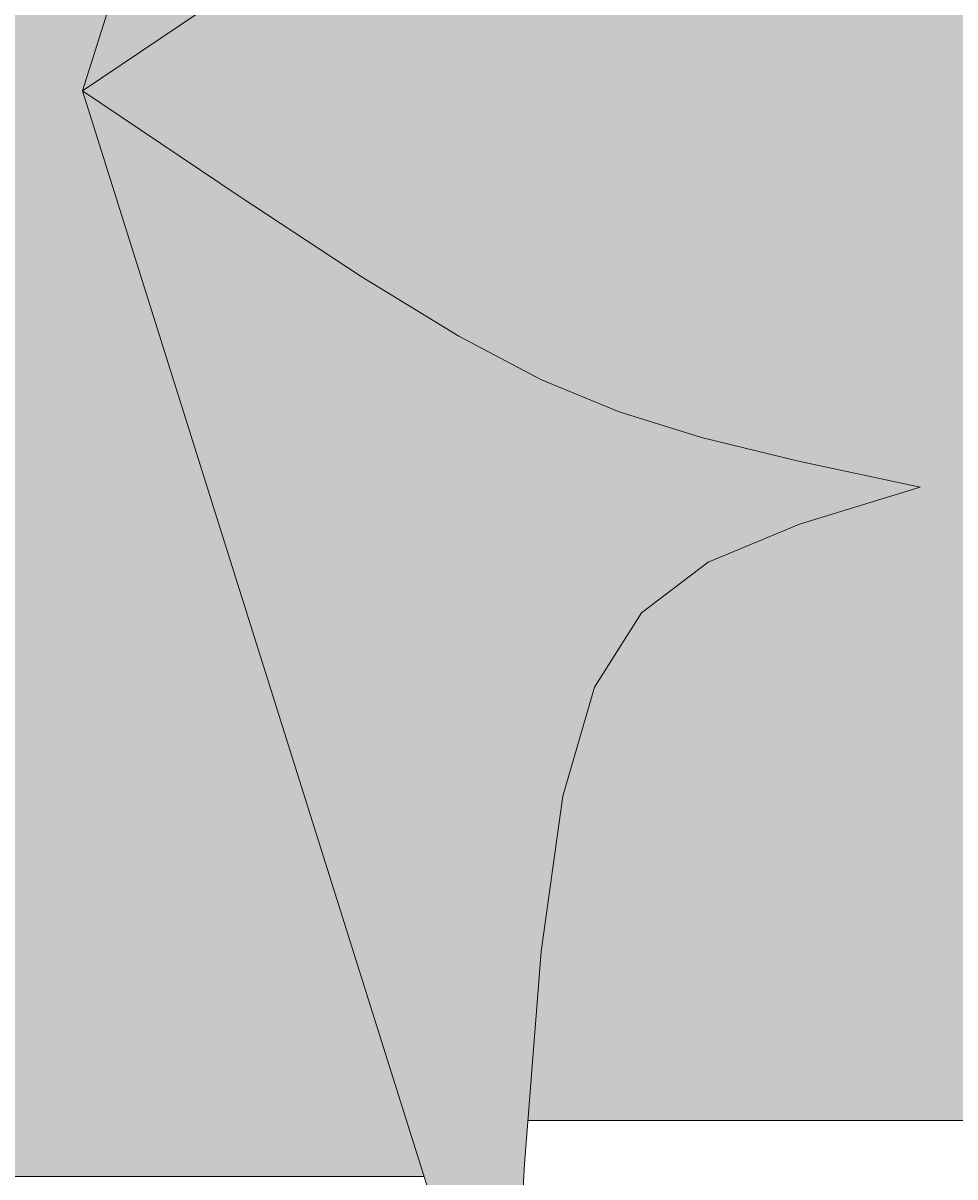
# Model space of a CAD drawing. Units: millimetres. Extents: x 27017497 to 27018854, y 7058029 to 7059154.
# Tile 82 of 91: x 27018341 to 27018362, y 7058503 to 7058530. Entities that reach past the tile are written whole.
import ezdxf

# ---------------------------------------------------------------- set-up
doc = ezdxf.new("R2010")
doc.units = ezdxf.units.MM
doc.layers.add('A-ANNO-DIMS', color=2, linetype='Continuous', lineweight=18)
doc.layers.add('A-FURN', color=8, linetype='Continuous', lineweight=18)
doc.layers.add('A-FURN-PATT', color=177, linetype='Continuous', lineweight=13, true_color=0x293189)
doc.styles.get("Standard").update_dxf_attribs({"font": 'arial.ttf'})
doc.dimstyles.get("Standard").update_dxf_attribs({"dimtxt": 0.18, "dimasz": 0.18, "dimexe": 0.18, "dimexo": 0.0625, "dimgap": 0.09, "dimtad": 0, "dimtih": 1, "dimtoh": 1, "dimdec": 4, "dimzin": 0, "dimdsep": 46, "dimtxsty": 'Standard', "dimcen": 0.09, "dimadec": 0, "dimazin": 0, "dimtfac": 1, "dimtdec": 4, "dimtofl": 0, "dimtmove": 0, "dimatfit": 3, "dimfxl": 1, "dimtolj": 1, "dimtzin": 0, "dimarcsym": 0})

# ---------------------------------------------------------------- blocks, each defined once
blk = doc.blocks.new('CAMMAT')
for p, q in [((0.68256, -0.51693), (0.68256, -0.76028)), ((0.05354, -0.5623), (-0.73116, -0.80928)), ((0.05354, -0.5623), (0.83824, -0.80928)), ((0.65, -0.82044), (0.65, -1.93))]:
    blk.add_line(p, q)
for points in [[(-0.17613, -1.04763), (-0.161, -0.97721), (-0.14737, -0.92096), (-0.13256, -0.87318), (-0.11386, -0.82818), (-0.0886, -0.78028), (-0.05407, -0.7238), (-0.00759, -0.65303), (0.05354, -0.5623)], [(0.28321, -1.04763), (0.26808, -0.97721), (0.25445, -0.92096), (0.23964, -0.87318), (0.22094, -0.82818), (0.19568, -0.78028), (0.16115, -0.7238), (0.11467, -0.65303), (0.05354, -0.5623)], [(0.83824, -0.80928), (0.67535, -0.81849), (0.55218, -0.82799), (0.46223, -0.84058), (0.39901, -0.85906), (0.356, -0.8862), (0.3267, -0.92482), (0.3046, -0.9777), (0.28321, -1.04763)]]:
    blk.add_lwpolyline(points)
blk = doc.blocks.new('*D48')
at = {"layer": 'A-ANNO-DIMS', "color": 0, "lineweight": -2, "transparency": 16777216}
for p, q in [((27018463.498, 7058622.912), (27017497.536, 7058622.912)), ((27017497.716, 7058622.732), (27017497.716, 7058357.753)), ((27017497.716, 7058092.41), (27017497.716, 7058357.389)), ((27018555.129, 7058092.23), (27017497.536, 7058092.23))]:
    blk.add_line(p, q, dxfattribs=at)
at = {"layer": 'A-ANNO-DIMS', "color": 0, "transparency": 16777216}
for points in [[(27017497.686, 7058622.732), (27017497.746, 7058622.732), (27017497.716, 7058622.912)], [(27017497.686, 7058092.41), (27017497.746, 7058092.41), (27017497.716, 7058092.23)]]:
    blk.add_solid(points, dxfattribs=at)
at = {"layer": 'Defpoints', "color": 0, "transparency": 16777216}
for p in [(27018463.561, 7058622.912), (27017497.716, 7058092.23), (27018555.192, 7058092.23)]:
    blk.add_point(p, dxfattribs=at)
at = {"layer": 'A-ANNO-DIMS', "color": 0, "transparency": 16777216, "insert": (27017497.716, 7058357.571), "char_height": 0.18, "attachment_point": 5}
blk.add_mtext('\\A1;530.7', dxfattribs=at)
blk = doc.blocks.new('*D50')
at = {"layer": 'A-ANNO-DIMS', "color": 0, "lineweight": -2, "transparency": 16777216}
for p, q in [((27018223.668, 7058580.912), (27018854.236, 7058580.912)), ((27018854.056, 7058580.732), (27018854.056, 7058511.344)), ((27018854.056, 7058441.592), (27018854.056, 7058510.98)), ((27018223.668, 7058441.412), (27018854.236, 7058441.412))]:
    blk.add_line(p, q, dxfattribs=at)
at = {"layer": 'A-ANNO-DIMS', "color": 0, "transparency": 16777216}
for points in [[(27018854.026, 7058580.732), (27018854.086, 7058580.732), (27018854.056, 7058580.912)], [(27018854.026, 7058441.592), (27018854.086, 7058441.592), (27018854.056, 7058441.412)]]:
    blk.add_solid(points, dxfattribs=at)
at = {"layer": 'Defpoints', "color": 0, "transparency": 16777216}
for p in [(27018223.606, 7058580.912), (27018223.606, 7058441.412), (27018854.056, 7058441.412)]:
    blk.add_point(p, dxfattribs=at)
at = {"layer": 'A-ANNO-DIMS', "color": 0, "transparency": 16777216, "insert": (27018854.056, 7058511.162), "char_height": 0.18, "attachment_point": 5}
blk.add_mtext('\\A1;139.5', dxfattribs=at)

msp = doc.modelspace()

# ---------------------------------------------------------------- hatches: boundary and pattern name
at = {"layer": 'A-FURN-PATT'}
h = msp.add_hatch(color=256, dxfattribs=at)
h.dxf.hatch_style = 1
h.paths.add_polyline_path([(27018398.067, 7058554.497, 0.414214), (27018396.474, 7058556.09), (27018352.018, 7058556.09), (27018352.202, 7058552.834), (27018352.581, 7058547.929), (27018353.082, 7058544.346), (27018353.818, 7058541.828), (27018354.899, 7058540.115), (27018356.437, 7058538.948), (27018358.543, 7058538.068), (27018361.329, 7058537.215), (27018358.524, 7058536.613), (27018356.284, 7058536.07), (27018354.381, 7058535.48), (27018352.588, 7058534.736), (27018350.68, 7058533.729), (27018348.431, 7058532.354), (27018345.612, 7058530.503), (27018341.998, 7058528.068), (27018345.612, 7058525.633), (27018348.431, 7058523.782), (27018350.68, 7058522.407), (27018352.588, 7058521.4), (27018354.381, 7058520.656), (27018356.284, 7058520.066), (27018358.524, 7058519.523), (27018361.329, 7058518.92), (27018358.543, 7058518.068), (27018356.437, 7058517.188), (27018354.899, 7058516.021), (27018353.818, 7058514.308), (27018353.082, 7058511.79), (27018352.581, 7058508.207), (27018352.28, 7058504.311), (27018396.474, 7058504.311, 0.414214), (27018398.067, 7058505.904)])
h.paths.add_polyline_path([(27018356.437, 7058538.948), (27018354.899, 7058540.115), (27018353.818, 7058541.828), (27018353.082, 7058544.346), (27018352.581, 7058547.929), (27018352.202, 7058552.834), (27018351.835, 7058559.322), (27018341.998, 7058528.068), (27018345.612, 7058530.503), (27018348.431, 7058532.354), (27018350.68, 7058533.729), (27018352.588, 7058534.736), (27018354.381, 7058535.48), (27018356.284, 7058536.07), (27018358.524, 7058536.613), (27018361.329, 7058537.215), (27018358.543, 7058538.068)])
h.paths.add_polyline_path([(27018358.543, 7058518.068), (27018361.329, 7058518.92), (27018358.524, 7058519.523), (27018356.284, 7058520.066), (27018354.381, 7058520.656), (27018352.588, 7058521.4), (27018350.68, 7058522.407), (27018348.431, 7058523.782), (27018345.612, 7058525.633), (27018341.998, 7058528.068), (27018351.835, 7058496.813), (27018352.202, 7058503.301), (27018352.581, 7058508.207), (27018353.082, 7058511.79), (27018353.818, 7058514.308), (27018354.899, 7058516.021), (27018356.437, 7058517.188)])
h.paths.add_polyline_path([(27018351.324, 7058557.699), (27018340.191, 7058557.699), (27018340.191, 7058503.014), (27018349.884, 7058503.014), (27018341.998, 7058528.068)])
h.paths.add_polyline_path([(27018340.191, 7058556.09), (27018323.983, 7058556.09, 0.414214), (27018322.39, 7058554.497), (27018322.39, 7058505.904, 0.414214), (27018323.983, 7058504.311), (27018340.191, 7058504.311)])
h.paths.add_polyline_path([(27018337.107, 7058532.051, -0.414214), (27018335.912, 7058530.856), (27018326.353, 7058530.856, -0.414214), (27018325.158, 7058532.051), (27018325.158, 7058553.51, -0.414214), (27018326.353, 7058554.705), (27018335.912, 7058554.705, -0.414214), (27018337.107, 7058553.51)], flags=0)
h.paths.add_polyline_path([(27018337.107, 7058527.914), (27018337.107, 7058506.454, -0.414214), (27018335.912, 7058505.259), (27018326.353, 7058505.259, -0.414214), (27018325.158, 7058506.454), (27018325.158, 7058527.914, -0.414214), (27018326.353, 7058529.109), (27018335.912, 7058529.109, -0.414214)], flags=0)
h.paths.add_polyline_path([(27018338.322, 7058577.2), (27018322.39, 7058577.2), (27018322.39, 7058557.285), (27018338.322, 7058557.285)])
h.paths.add_polyline_path([(27018323.748, 7058567.284, -1), (27018335.697, 7058567.284, -1)], flags=16)
h.paths.add_polyline_path([(27018326.023, 7058567.284, -1), (27018333.423, 7058567.284, -1)], flags=0)
h.paths.add_polyline_path([(27018338.322, 7058503.116), (27018322.39, 7058503.116), (27018322.39, 7058483.201), (27018338.322, 7058483.201)])
h.paths.add_polyline_path([(27018335.697, 7058493.391, -1), (27018323.748, 7058493.391, -1)], flags=16)
h.paths.add_polyline_path([(27018333.423, 7058493.391, -1), (27018326.023, 7058493.391, -1)], flags=0)
h.paths.add_polyline_path([(27018337.107, 7058527.914, 0.414214), (27018335.912, 7058529.109), (27018326.353, 7058529.109, 0.414214), (27018325.158, 7058527.914), (27018325.158, 7058506.454, 0.414214), (27018326.353, 7058505.259), (27018335.912, 7058505.259, 0.414214), (27018337.107, 7058506.454)], flags=16)
h.paths.add_polyline_path([(27018337.107, 7058553.51, 0.414214), (27018335.912, 7058554.705), (27018326.353, 7058554.705, 0.414214), (27018325.158, 7058553.51), (27018325.158, 7058532.051, 0.414214), (27018326.353, 7058530.856), (27018335.912, 7058530.856, 0.414214), (27018337.107, 7058532.051)], flags=16)

# ---------------------------------------------------------------- block references
at = {"layer": 'A-FURN', "xscale": -39.82996475819422, "yscale": 39.82996475819422, "zscale": 39.82996475819422, "rotation": 90}
msp.add_blockref('CAMMAT', (27018319.602, 7058530.2), dxfattribs=at)

# ---------------------------------------------------------------- dimensions: what is measured, and where the dimension line sits
at = {"layer": 'A-ANNO-DIMS'}
for base, p1, p2, picture, middle in [((27017497.716, 7058092.23), (27018463.561, 7058622.912), (27018555.192, 7058092.23), '*D48', (27017497.716, 7058357.571)), ((27018854.056, 7058441.412), (27018223.606, 7058580.912), (27018223.606, 7058441.412), '*D50', (27018854.056, 7058511.162))]:
    dim = msp.add_linear_dim(base=base, p1=p1, p2=p2, angle=90, dimstyle='Standard', override={"dimdec": 1, "dimlfac": 1, "dimrnd": 0, "dimzin": 0, "dimdsep": 46, "dimlunit": 2}, dxfattribs=at)
    dim.commit()
    dim.dimension.update_dxf_attribs({"geometry": picture, "text_midpoint": middle})

doc.saveas('drawing.dxf')
